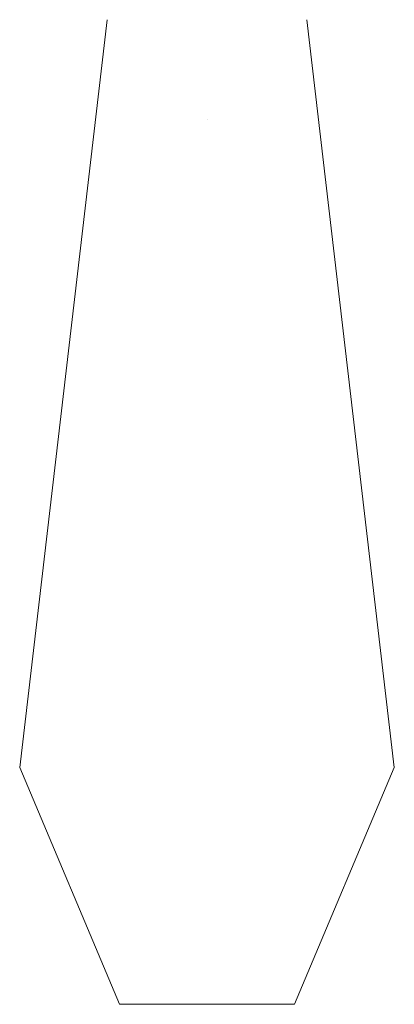
# Model space of a CAD drawing. Units: millimetres. Extents: x 502 to 562, y 419 to 577.
import ezdxf

# ---------------------------------------------------------------- set-up
doc = ezdxf.new("R2010")
doc.units = ezdxf.units.MM
doc.layers.add('M-CONS', color=8, linetype='Continuous', lineweight=18)

msp = doc.modelspace()

# ---------------------------------------------------------------- linework, layer by layer
at = {"layer": 'M-CONS'}
for p, q in [((515.7, 576.53, 12), (501.7, 456.53, 12)), ((561.7, 456.53, 12), (547.7, 576.53, 12)), ((531.7, 560.53, 12), (531.7, 560.53, 15)), ((517.7, 418.53, 34), (501.7, 456.53, 34)), ((545.7, 418.53, 34), (561.7, 456.53, 34)), ((561.7, 456.53, 40), (561.7, 456.53, 34)), ((517.7, 418.53, 34), (545.7, 418.53, 34))]:
    msp.add_line(p, q, dxfattribs=at)

doc.saveas('drawing.dxf')
